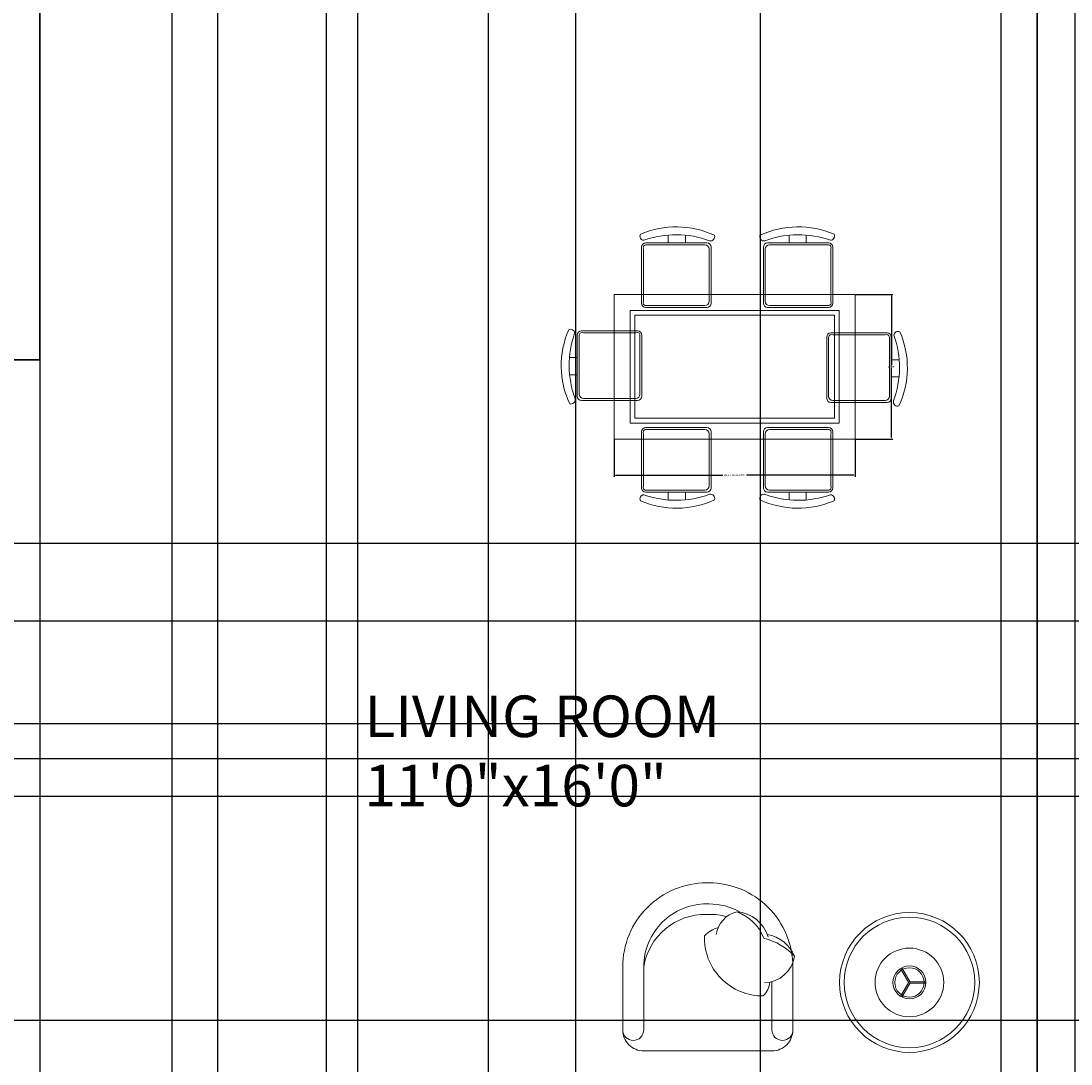
# Model space of a CAD drawing. Units: inches. Extents: x 1861 to 2564, y 1482 to 2317.
# Tile 6 of 11: x 2090 to 2217, y 2018 to 2143. Entities that reach past the tile are written whole.
import ezdxf

# ---------------------------------------------------------------- set-up
doc = ezdxf.new("R2010")
doc.units = ezdxf.units.IN
for name, color, linetype, lineweight in [('A-ANNO-DIMS', 2, 'Continuous', 18), ('A-AREA-IDEN', 7, 'Continuous', 18), ('A-FURN', 8, 'Continuous', 13), ('A-WALL', 7, 'Continuous', 35)]:
    doc.layers.add(name, color=color, linetype=linetype, lineweight=lineweight)
doc.styles.get("Standard").update_dxf_attribs({"font": 'arial.ttf'})
doc.dimstyles.get("Standard").update_dxf_attribs({"dimtxt": 0.18, "dimasz": 0.18, "dimexe": 0.18, "dimexo": 0.0625, "dimgap": 0.09, "dimtad": 0, "dimtih": 1, "dimtoh": 1, "dimdec": 4, "dimzin": 0, "dimdsep": 46, "dimtxsty": 'Standard', "dimcen": 0.09, "dimadec": 0, "dimazin": 0, "dimtfac": 1, "dimtdec": 4, "dimtofl": 0, "dimtmove": 0, "dimatfit": 3, "dimfxl": 1, "dimtolj": 1, "dimtzin": 0, "dimarcsym": 0})

# ---------------------------------------------------------------- blocks, each defined once
blk = doc.blocks.new('TABLE-SIDE-ROUND')
at = {"ltscale": 0.03}
for p, q in [((8.34, 8.45), (9.33, 10.16)), ((8.49, 8.36), (9.48, 10.08)), ((8.41, 8.5), (6.44, 8.5)), ((8.41, 8.32), (6.44, 8.32)), ((8.34, 8.36), (9.33, 6.65)), ((8.49, 8.45), (9.48, 6.74))]:
    blk.add_line(p, q, dxfattribs=at)
for radius in [8.41, 4.13, 1.98, 1.77]:
    blk.add_circle((8.41, 8.41), radius, dxfattribs=at)
blk.add_circle((8.41, 8.41), 7.85)
blk = doc.blocks.new('CHAIR-LOUNGE')
at = {"ltscale": 0.03}
blk.add_lwpolyline([(10.44, 0), (18.15, 0, 0.414214), (20.68, 2.53), (20.68, 10.11, 0.414214), (10.57, 20.22), (10.44, 20.22), (10.32, 20.22, 0.414214), (0.21, 10.11), (0.21, 2.53, 0.414214), (2.73, 0), (10.44, 0)], format="xyb", dxfattribs=at)
for points in [[(6.55, 16.69, -0.130591), (10.32, 17.69), (10.44, 17.69)], [(18.15, 10.11, 0.414214), (10.57, 17.69), (10.44, 17.69)], [(0, 11.38, -0.14773), (3.69, 13.56, -0.213343), (6.95, 16.74, -0.178662)], [(3.18, 13.73, -0.306663), (6.95, 16.74, -0.30633), (9.42, 13.99, 0.872847)], [(8.16, 16.16, -0.072384), (10.32, 16.43), (10.44, 16.43)], [(18.15, 10.11, 0.372719), (10.57, 16.43), (10.44, 16.43)], [(3.62, 8.2, -0.356772), (0, 11.38, -0.249542), (3.28, 14.01, 9.61688)], [(2.98, 8.28, 0.165541), (3.77, 6.61, 0.425989), (10.86, 13.85, 0.121523), (9.18, 14.84, -7.115464)], [(18.15, 10.11), (18.15, 2.53, 0.414214), (19.42, 1.26), (19.42, 1.26, 0.414214), (20.68, 2.53)], [(2.73, 8.34), (2.73, 2.53, -0.414214), (1.47, 1.26), (1.47, 1.26, -0.414214), (0.21, 2.53)]]:
    blk.add_lwpolyline(points, format="xyb")
blk = doc.blocks.new('TABLE-DINING-RECT')
for points in [[(0, 17.4), (29.01, 17.4), (29.01, 0), (0, 0)], [(0, 17.4), (29.01, 17.4), (29.01, 0), (0, 0)], [(1.93, 15.47), (27.08, 15.47), (27.08, 1.93), (1.93, 1.93)], [(1.93, 15.47), (27.08, 15.47), (27.08, 1.93), (1.93, 1.93)], [(2.51, 14.89), (26.5, 14.89), (26.5, 2.51), (2.51, 2.51)], [(2.51, 14.89), (26.5, 14.89), (26.5, 2.51), (2.51, 2.51)]]:
    blk.add_lwpolyline(points, close=True)
blk = doc.blocks.new('*D32')
at = {"layer": 'A-ANNO-DIMS', "color": 0, "lineweight": -2, "transparency": 16777216}
for p, q in [((2161.83, 2092.8), (2161.83, 2088.34)), ((2190.84, 2092.8), (2190.84, 2088.34)), ((2162.01, 2088.52), (2174.9, 2088.52)), ((2190.66, 2088.52), (2177.77, 2088.52))]:
    blk.add_line(p, q, dxfattribs=at)
at = {"layer": 'A-ANNO-DIMS', "color": 0, "transparency": 16777216}
for points in [[(2162.01, 2088.55), (2162.01, 2088.49), (2161.83, 2088.52)], [(2190.66, 2088.55), (2190.66, 2088.49), (2190.84, 2088.52)]]:
    blk.add_solid(points, dxfattribs=at)
at = {"layer": 'Defpoints', "color": 0, "transparency": 16777216}
for p in [(2161.83, 2092.87), (2190.84, 2092.87), (2190.84, 2088.52)]:
    blk.add_point(p, dxfattribs=at)
at = {"layer": 'A-ANNO-DIMS', "color": 0, "transparency": 16777216, "insert": (2176.33, 2088.52), "char_height": 0.18, "attachment_point": 5}
blk.add_mtext('\\A1;DINING TABLE 29 TYP.', dxfattribs=at)
blk = doc.blocks.new('*D33')
at = {"layer": 'A-ANNO-DIMS', "color": 0, "lineweight": -2, "transparency": 16777216}
for p, q in [((2190.9, 2110.27), (2195.37, 2110.27)), ((2195.19, 2110.09), (2195.19, 2101.75)), ((2195.19, 2093.05), (2195.19, 2101.39)), ((2190.9, 2092.87), (2195.37, 2092.87))]:
    blk.add_line(p, q, dxfattribs=at)
at = {"layer": 'A-ANNO-DIMS', "color": 0, "transparency": 16777216}
for points in [[(2195.16, 2110.09), (2195.22, 2110.09), (2195.19, 2110.27)], [(2195.16, 2093.05), (2195.22, 2093.05), (2195.19, 2092.87)]]:
    blk.add_solid(points, dxfattribs=at)
at = {"layer": 'Defpoints', "color": 0, "transparency": 16777216}
for p in [(2190.84, 2110.27), (2195.19, 2110.27), (2190.84, 2092.87)]:
    blk.add_point(p, dxfattribs=at)
at = {"layer": 'A-ANNO-DIMS', "color": 0, "transparency": 16777216, "insert": (2195.19, 2101.57), "char_height": 0.18, "attachment_point": 5}
blk.add_mtext('\\A1;17 TYP.', dxfattribs=at)
blk = doc.blocks.new('*D36')
at = {"layer": 'A-ANNO-DIMS', "color": 0, "lineweight": -2, "transparency": 16777216}
for p, q in [((2092.74, 2250.82), (2092.74, 1545.6)), ((2127.18, 2250.82), (2127.18, 1545.6)), ((2092.92, 1545.78), (2109.5, 1545.78)), ((2127, 1545.78), (2110.43, 1545.78))]:
    blk.add_line(p, q, dxfattribs=at)
at = {"layer": 'A-ANNO-DIMS', "color": 0, "transparency": 16777216}
for points in [[(2092.92, 1545.81), (2092.92, 1545.75), (2092.74, 1545.78)], [(2127, 1545.81), (2127, 1545.75), (2127.18, 1545.78)]]:
    blk.add_solid(points, dxfattribs=at)
at = {"layer": 'Defpoints', "color": 0, "transparency": 16777216}
for p in [(2092.74, 2250.89), (2127.18, 2250.89), (2127.18, 1545.78)]:
    blk.add_point(p, dxfattribs=at)
at = {"layer": 'A-ANNO-DIMS', "color": 0, "transparency": 16777216, "insert": (2109.96, 1545.78), "char_height": 0.18, "attachment_point": 5}
blk.add_mtext('\\A1;34.445', dxfattribs=at)
blk = doc.blocks.new('*D52')
at = {"layer": 'A-ANNO-DIMS', "color": 0, "lineweight": -2, "transparency": 16777216}
for p, q in [((2179.39, 2154.82), (2179.39, 1545.6)), ((2208.37, 2154.82), (2208.37, 1545.6)), ((2179.57, 1545.78), (2193.49, 1545.78)), ((2208.19, 1545.78), (2194.28, 1545.78))]:
    blk.add_line(p, q, dxfattribs=at)
at = {"layer": 'A-ANNO-DIMS', "color": 0, "transparency": 16777216}
for points in [[(2179.57, 1545.81), (2179.57, 1545.75), (2179.39, 1545.78)], [(2208.19, 1545.81), (2208.19, 1545.75), (2208.37, 1545.78)]]:
    blk.add_solid(points, dxfattribs=at)
at = {"layer": 'Defpoints', "color": 0, "transparency": 16777216}
for p in [(2179.39, 2154.89), (2208.37, 2154.89), (2208.37, 1545.78)]:
    blk.add_point(p, dxfattribs=at)
at = {"layer": 'A-ANNO-DIMS', "color": 0, "transparency": 16777216, "insert": (2193.88, 1545.78), "char_height": 0.18, "attachment_point": 5}
blk.add_mtext('\\A1;28.98', dxfattribs=at)
blk = doc.blocks.new('*D55')
at = {"layer": 'A-ANNO-DIMS', "color": 0, "lineweight": -2, "transparency": 16777216}
for p, q in [((2114.18, 1853.45), (2114.18, 2290.37)), ((2114.36, 2290.19), (2130, 2290.19)), ((2146.56, 2290.19), (2130.92, 2290.19)), ((2146.74, 1853.45), (2146.74, 2290.37))]:
    blk.add_line(p, q, dxfattribs=at)
at = {"layer": 'A-ANNO-DIMS', "color": 0, "transparency": 16777216}
for points in [[(2114.36, 2290.22), (2114.36, 2290.16), (2114.18, 2290.19)], [(2146.56, 2290.22), (2146.56, 2290.16), (2146.74, 2290.19)]]:
    blk.add_solid(points, dxfattribs=at)
at = {"layer": 'Defpoints', "color": 0, "transparency": 16777216}
for p in [(2146.74, 2290.19), (2114.18, 1853.39), (2146.74, 1853.39)]:
    blk.add_point(p, dxfattribs=at)
at = {"layer": 'A-ANNO-DIMS', "color": 0, "transparency": 16777216, "insert": (2130.46, 2290.19), "char_height": 0.18, "attachment_point": 5}
blk.add_mtext('\\A1;32.564', dxfattribs=at)
blk = doc.blocks.new('*D61')
at = {"layer": 'A-ANNO-DIMS', "color": 0, "lineweight": -2, "transparency": 16777216}
for p, q in [((2008.8, 2080.33), (2537.22, 2080.33)), ((2537.04, 2080.15), (2537.04, 2069.66)), ((2537.04, 2058.82), (2537.04, 2069.3)), ((2008.8, 2058.64), (2537.22, 2058.64))]:
    blk.add_line(p, q, dxfattribs=at)
at = {"layer": 'A-ANNO-DIMS', "color": 0, "transparency": 16777216}
for points in [[(2537.01, 2080.15), (2537.07, 2080.15), (2537.04, 2080.33)], [(2537.01, 2058.82), (2537.07, 2058.82), (2537.04, 2058.64)]]:
    blk.add_solid(points, dxfattribs=at)
at = {"layer": 'Defpoints', "color": 0, "transparency": 16777216}
for p in [(2008.74, 2080.33), (2537.04, 2080.33), (2008.74, 2058.64)]:
    blk.add_point(p, dxfattribs=at)
at = {"layer": 'A-ANNO-DIMS', "color": 0, "transparency": 16777216, "insert": (2537.04, 2069.48), "char_height": 0.18, "attachment_point": 5}
blk.add_mtext('\\A1;21.693', dxfattribs=at)
blk = doc.blocks.new('*D62')
at = {"layer": 'A-ANNO-DIMS', "color": 0, "lineweight": -2, "transparency": 16777216}
for p, q in [((2108.68, 1781.45), (2108.68, 2290.37)), ((2108.86, 2290.19), (2119.46, 2290.19)), ((2130.84, 2290.19), (2120.25, 2290.19)), ((2131.02, 1781.45), (2131.02, 2290.37))]:
    blk.add_line(p, q, dxfattribs=at)
at = {"layer": 'A-ANNO-DIMS', "color": 0, "transparency": 16777216}
for points in [[(2108.86, 2290.22), (2108.86, 2290.16), (2108.68, 2290.19)], [(2130.84, 2290.22), (2130.84, 2290.16), (2131.02, 2290.19)]]:
    blk.add_solid(points, dxfattribs=at)
at = {"layer": 'Defpoints', "color": 0, "transparency": 16777216}
for p in [(2131.02, 2290.19), (2108.68, 1781.39), (2131.02, 1781.39)]:
    blk.add_point(p, dxfattribs=at)
at = {"layer": 'A-ANNO-DIMS', "color": 0, "transparency": 16777216, "insert": (2119.85, 2290.19), "char_height": 0.18, "attachment_point": 5}
blk.add_mtext('\\A1;22.34', dxfattribs=at)
blk = doc.blocks.new('*D64')
at = {"layer": 'A-ANNO-DIMS', "color": 0, "lineweight": -2, "transparency": 16777216}
for p, q in [((2497.68, 2070.96), (1892.76, 2070.96)), ((1892.94, 2070.78), (1892.94, 2062.85)), ((1892.94, 2054.57), (1892.94, 2062.49)), ((2497.68, 2054.39), (1892.76, 2054.39))]:
    blk.add_line(p, q, dxfattribs=at)
at = {"layer": 'A-ANNO-DIMS', "color": 0, "transparency": 16777216}
for points in [[(1892.91, 2070.78), (1892.97, 2070.78), (1892.94, 2070.96)], [(1892.91, 2054.57), (1892.97, 2054.57), (1892.94, 2054.39)]]:
    blk.add_solid(points, dxfattribs=at)
at = {"layer": 'Defpoints', "color": 0, "transparency": 16777216}
for p in [(2497.74, 2070.96), (1892.94, 2054.39), (2497.74, 2054.39)]:
    blk.add_point(p, dxfattribs=at)
at = {"layer": 'A-ANNO-DIMS', "color": 0, "transparency": 16777216, "insert": (1892.94, 2062.67), "char_height": 0.18, "attachment_point": 5}
blk.add_mtext('\\A1;16.57', dxfattribs=at)
blk = doc.blocks.new('*D65')
at = {"layer": 'A-ANNO-DIMS', "color": 0, "lineweight": -2, "transparency": 16777216}
for p, q in [((2497.68, 2049.89), (1892.76, 2049.89)), ((1892.94, 2049.71), (1892.94, 2036.58)), ((1892.94, 2023.09), (1892.94, 2036.22)), ((2497.68, 2022.91), (1892.76, 2022.91))]:
    blk.add_line(p, q, dxfattribs=at)
at = {"layer": 'A-ANNO-DIMS', "color": 0, "transparency": 16777216}
for points in [[(1892.91, 2049.71), (1892.97, 2049.71), (1892.94, 2049.89)], [(1892.91, 2023.09), (1892.97, 2023.09), (1892.94, 2022.91)]]:
    blk.add_solid(points, dxfattribs=at)
at = {"layer": 'Defpoints', "color": 0, "transparency": 16777216}
for p in [(2497.74, 2049.89), (1892.94, 2022.91), (2497.74, 2022.91)]:
    blk.add_point(p, dxfattribs=at)
at = {"layer": 'A-ANNO-DIMS', "color": 0, "transparency": 16777216, "insert": (1892.94, 2036.4), "char_height": 0.18, "attachment_point": 5}
blk.add_mtext('\\A1;26.973', dxfattribs=at)
blk = doc.blocks.new('*D68')
at = {"layer": 'A-ANNO-DIMS', "color": 0, "lineweight": -2, "transparency": 16777216}
for p, q in [((2157.24, 1794.95), (2157.24, 2290.37)), ((2157.42, 2290.19), (2184.66, 2290.19)), ((2212.56, 2290.19), (2185.31, 2290.19)), ((2212.74, 1794.95), (2212.74, 2290.37))]:
    blk.add_line(p, q, dxfattribs=at)
at = {"layer": 'A-ANNO-DIMS', "color": 0, "transparency": 16777216}
for points in [[(2157.42, 2290.22), (2157.42, 2290.16), (2157.24, 2290.19)], [(2212.56, 2290.22), (2212.56, 2290.16), (2212.74, 2290.19)]]:
    blk.add_solid(points, dxfattribs=at)
at = {"layer": 'Defpoints', "color": 0, "transparency": 16777216}
for p in [(2212.74, 2290.19), (2157.24, 1794.89), (2212.74, 1794.89)]:
    blk.add_point(p, dxfattribs=at)
at = {"layer": 'A-ANNO-DIMS', "color": 0, "transparency": 16777216, "insert": (2184.99, 2290.19), "char_height": 0.18, "attachment_point": 5}
blk.add_mtext('\\A1;55.5', dxfattribs=at)
blk = doc.blocks.new('*D71')
at = {"layer": 'A-ANNO-DIMS', "color": 0, "lineweight": -2, "transparency": 16777216}
for p, q in [((2212.74, 2250.82), (2212.74, 1545.6)), ((2217.24, 2250.82), (2217.24, 1545.6)), ((2212.92, 1545.78), (2214.73, 1545.78)), ((2217.06, 1545.78), (2215.25, 1545.78))]:
    blk.add_line(p, q, dxfattribs=at)
at = {"layer": 'A-ANNO-DIMS', "color": 0, "transparency": 16777216}
for points in [[(2212.92, 1545.81), (2212.92, 1545.75), (2212.74, 1545.78)], [(2217.06, 1545.81), (2217.06, 1545.75), (2217.24, 1545.78)]]:
    blk.add_solid(points, dxfattribs=at)
at = {"layer": 'Defpoints', "color": 0, "transparency": 16777216}
for p in [(2212.74, 2250.89), (2217.24, 2250.89), (2217.24, 1545.78)]:
    blk.add_point(p, dxfattribs=at)
at = {"layer": 'A-ANNO-DIMS', "color": 0, "transparency": 16777216, "insert": (2214.99, 1545.78), "char_height": 0.18, "attachment_point": 5}
blk.add_mtext('\\A1;4.5', dxfattribs=at)

msp = doc.modelspace()

# ---------------------------------------------------------------- linework, layer by layer
at = {"layer": 'A-FURN'}
for points in [[(2165.4177, 2116.7864, -0.17580919), (2173.3194, 2116.7265, 0.57839206), (2173.918, 2117.3847, 0.21452438), (2164.9987, 2117.5044, 0.55201397), (2165.4177, 2116.7864, -0.06507904)], [(2165.4177, 2116.7861, -0.17580919), (2173.3194, 2116.7262, 0.57839206), (2173.9181, 2117.3844, 0.21452438), (2164.9987, 2117.5041, 0.55201397), (2165.4177, 2116.7861, -0.06507904)], [(2179.9716, 2116.7265, -0.57839206), (2179.373, 2117.3847, -0.21452438), (2188.2924, 2117.5044, -0.55201397), (2187.8733, 2116.7864, 0.1758092), (2179.9716, 2116.7265)], [(2179.9717, 2116.7262, -0.57839206), (2179.373, 2117.3844, -0.21452438), (2188.2924, 2117.5041, -0.55201397), (2187.8734, 2116.7861, 0.1758092), (2179.9717, 2116.7262)], [(2170.4075, 2116.4692), (2170.4075, 2117.397, -0.06475861)], [(2170.4076, 2116.4689), (2170.4076, 2117.3967, -0.06475861)], [(2182.8835, 2116.4692), (2182.8835, 2117.397, 0.06475861)], [(2182.8835, 2116.4689), (2182.8835, 2117.3967, 0.06475861)], [(2172.9842, 2116.4692), (2165.6485, 2116.4692, 0.41421356), (2165.1353, 2115.956), (2165.1353, 2109.211, 0.41421356), (2165.6485, 2108.6978), (2172.9842, 2108.6978, 0.41421356), (2173.4974, 2109.211), (2173.4974, 2115.956, 0.41421356), (2172.9842, 2116.4692)], [(2172.9842, 2116.4689), (2165.6485, 2116.4689, 0.41421356), (2165.1353, 2115.9557), (2165.1353, 2109.2107, 0.41421356), (2165.6485, 2108.6975), (2172.9842, 2108.6975, 0.41421356), (2173.4974, 2109.2107), (2173.4974, 2115.9557, 0.41421356), (2172.9842, 2116.4689)], [(2187.6425, 2116.4692, -0.41421356), (2188.1558, 2115.956), (2188.1558, 2109.211, -0.41421356), (2187.6425, 2108.6978), (2180.3069, 2108.6978, -0.41421356), (2179.7937, 2109.211), (2179.7937, 2115.956, -0.41421356), (2180.3069, 2116.4692), (2187.6425, 2116.4692)], [(2187.6426, 2116.4689, -0.41421356), (2188.1558, 2115.9557), (2188.1558, 2109.2107, -0.41421356), (2187.6426, 2108.6975), (2180.3069, 2108.6975, -0.41421356), (2179.7937, 2109.2107), (2179.7937, 2115.9557, -0.41421356), (2180.3069, 2116.4689), (2187.6426, 2116.4689)], [(2157.151, 2097.7049, -0.57839206), (2156.4928, 2097.1063, -0.21452438), (2156.3731, 2106.0257, -0.55201397), (2157.0912, 2105.6066, 0.17580937), (2157.151, 2097.7049)], [(2157.151, 2097.7046, -0.57839206), (2156.4928, 2097.106, -0.21452438), (2156.3731, 2106.0254, -0.55201397), (2157.0912, 2105.6063, 0.17580937), (2157.151, 2097.7046)], [(2157.4083, 2105.3759, -0.41421356), (2157.9215, 2105.8891), (2164.6665, 2105.8891, -0.41421356), (2165.1798, 2105.3759), (2165.1798, 2098.0402, -0.41421356), (2164.6665, 2097.527), (2157.9215, 2097.527, -0.41421356), (2157.4083, 2098.0402), (2157.4083, 2105.3759)], [(2157.4083, 2105.3755, -0.41421356), (2157.9216, 2105.8888), (2164.6666, 2105.8888, -0.41421356), (2165.1798, 2105.3755), (2165.1798, 2098.0399, -0.41421356), (2164.6666, 2097.5267), (2157.9216, 2097.5267, -0.41421356), (2157.4083, 2098.0399), (2157.4083, 2105.3755)], [(2195.1836, 2105.1246, 0.41421356), (2194.6704, 2105.6378), (2187.9254, 2105.6378, 0.41421356), (2187.4122, 2105.1246), (2187.4122, 2097.7889, 0.41421356), (2187.9254, 2097.2757), (2194.6704, 2097.2757, 0.41421356), (2195.1836, 2097.7889), (2195.1836, 2105.1246)], [(2195.1836, 2105.1243, 0.41421356), (2194.6704, 2105.6375), (2187.9254, 2105.6375, 0.41421356), (2187.4122, 2105.1243), (2187.4122, 2097.7886, 0.41421356), (2187.9254, 2097.2754), (2194.6704, 2097.2754, 0.41421356), (2195.1836, 2097.7886), (2195.1836, 2105.1243)], [(2195.5007, 2105.3554, -0.17580919), (2195.4409, 2097.4537, 0.57839206), (2196.0991, 2096.8551, 0.21452438), (2196.2188, 2105.7744, 0.55201397), (2195.5007, 2105.3554, -0.06507904)], [(2195.5008, 2105.3551, -0.17580919), (2195.4409, 2097.4534, 0.57839206), (2196.0991, 2096.8548, 0.21452438), (2196.2188, 2105.7741, 0.55201397), (2195.5008, 2105.3551, -0.06507904)], [(2157.4083, 2100.6168), (2156.4806, 2100.6168, 0.06475861)], [(2157.4083, 2100.6165), (2156.4806, 2100.6165, 0.06475861)], [(2195.1836, 2100.3656), (2196.1113, 2100.3656, -0.06475861)], [(2195.1836, 2100.3653), (2196.1114, 2100.3653, -0.06475861)], [(2172.9842, 2086.486), (2165.6485, 2086.486, -0.41421356), (2165.1353, 2086.9992), (2165.1353, 2093.7442, -0.41421356), (2165.6485, 2094.2574), (2172.9842, 2094.2574, -0.41421356), (2173.4974, 2093.7442), (2173.4974, 2086.9992, -0.41421356), (2172.9842, 2086.486)], [(2172.9842, 2086.4857), (2165.6485, 2086.4857, -0.41421356), (2165.1353, 2086.9989), (2165.1353, 2093.7439, -0.41421356), (2165.6485, 2094.2571), (2172.9842, 2094.2571, -0.41421356), (2173.4974, 2093.7439), (2173.4974, 2086.9989, -0.41421356), (2172.9842, 2086.4857)], [(2187.6425, 2086.486, 0.41421356), (2188.1558, 2086.9992), (2188.1558, 2093.7442, 0.41421356), (2187.6425, 2094.2574), (2180.3069, 2094.2574, 0.41421356), (2179.7937, 2093.7442), (2179.7937, 2086.9992, 0.41421356), (2180.3069, 2086.486), (2187.6425, 2086.486)], [(2187.6426, 2086.4857, 0.41421356), (2188.1558, 2086.9989), (2188.1558, 2093.7439, 0.41421356), (2187.6426, 2094.2571), (2180.3069, 2094.2571, 0.41421356), (2179.7937, 2093.7439), (2179.7937, 2086.9989, 0.41421356), (2180.3069, 2086.4857), (2187.6426, 2086.4857)], [(2173.3194, 2086.2287, -0.57839206), (2173.918, 2085.5705, -0.21452438), (2164.9987, 2085.4508, -0.55201397), (2165.4177, 2086.1689, 0.17580929), (2173.3194, 2086.2287)], [(2173.3194, 2086.2284, -0.57839206), (2173.9181, 2085.5702, -0.21452438), (2164.9987, 2085.4505, -0.55201397), (2165.4177, 2086.1686, 0.17580929), (2173.3194, 2086.2284)], [(2170.4075, 2086.486), (2170.4075, 2085.5583, 0.06475861)], [(2170.4076, 2086.4857), (2170.4076, 2085.558, 0.06475861)], [(2187.8733, 2086.1689, -0.17580928), (2179.9716, 2086.2287, 0.57839206), (2179.373, 2085.5705, 0.21452438), (2188.2924, 2085.4508, 0.55201397), (2187.8733, 2086.1689, -0.06507904)], [(2187.8734, 2086.1686, -0.17580928), (2179.9717, 2086.2284, 0.57839206), (2179.373, 2085.5702, 0.21452438), (2188.2924, 2085.4505, 0.55201397), (2187.8734, 2086.1686, -0.06507904)], [(2182.8835, 2086.486), (2182.8835, 2085.5583, -0.06475861)], [(2182.8835, 2086.4857), (2182.8835, 2085.558, -0.06475861)]]:
    msp.add_lwpolyline(points, format="xyb", dxfattribs=at)
for points in [[(2168.3542, 2117.4138), (2168.3542, 2116.4692)], [(2168.3542, 2117.4135), (2168.3542, 2116.4689)], [(2184.9369, 2117.4138), (2184.9369, 2116.4692)], [(2184.9369, 2117.4135), (2184.9369, 2116.4689)], [(2156.4637, 2102.6702), (2157.4083, 2102.6702)], [(2156.4637, 2102.6699), (2157.4083, 2102.6699)], [(2196.1282, 2102.419), (2195.1836, 2102.419)], [(2196.1282, 2102.4187), (2195.1836, 2102.4187)], [(2168.3542, 2085.5414), (2168.3542, 2086.486)], [(2168.3542, 2085.5411), (2168.3542, 2086.4857)], [(2184.9369, 2085.5414), (2184.9369, 2086.486)], [(2184.9369, 2085.5411), (2184.9369, 2086.4857)]]:
    msp.add_lwpolyline(points, dxfattribs=at)
for points in [[(2165.6516, 2116.238), (2172.753, 2116.238, -0.41421356), (2173.2662, 2115.7248), (2173.2662, 2109.4422, -0.41421356), (2172.753, 2108.929), (2165.6516, 2108.929, -0.51206948), (2165.3665, 2109.4422), (2165.3665, 2115.7248, -0.51206948)], [(2165.6516, 2116.2377), (2172.753, 2116.2377, -0.41421356), (2173.2662, 2115.7245), (2173.2662, 2109.4419, -0.41421356), (2172.753, 2108.9287), (2165.6516, 2108.9287, -0.51206948), (2165.3665, 2109.4419), (2165.3665, 2115.7245, -0.51206948)], [(2187.6394, 2116.238), (2180.5381, 2116.238, 0.41421356), (2180.0249, 2115.7248), (2180.0249, 2109.4422, 0.41421356), (2180.5381, 2108.929), (2187.6394, 2108.929, 0.51206948), (2187.9246, 2109.4422), (2187.9246, 2115.7248, 0.51206948)], [(2187.6395, 2116.2377), (2180.5381, 2116.2377, 0.41421356), (2180.0249, 2115.7245), (2180.0249, 2109.4419, 0.41421356), (2180.5381, 2108.9287), (2187.6395, 2108.9287, 0.51206948), (2187.9246, 2109.4419), (2187.9246, 2115.7245, 0.51206948)], [(2157.6395, 2105.3727), (2157.6395, 2098.2714, 0.41421356), (2158.1527, 2097.7582), (2164.4353, 2097.7582, 0.41421356), (2164.9486, 2098.2714), (2164.9486, 2105.3727, 0.51206948), (2164.4353, 2105.6579), (2158.1527, 2105.6579, 0.51206948)], [(2157.6395, 2105.3724), (2157.6395, 2098.2711, 0.41421356), (2158.1528, 2097.7579), (2164.4354, 2097.7579, 0.41421356), (2164.9486, 2098.2711), (2164.9486, 2105.3724, 0.51206948), (2164.4354, 2105.6576), (2158.1528, 2105.6576, 0.51206948)], [(2194.9524, 2105.1215), (2194.9524, 2098.0202, -0.41421356), (2194.4392, 2097.5069), (2188.1566, 2097.5069, -0.41421356), (2187.6434, 2098.0202), (2187.6434, 2105.1215, -0.51206948), (2188.1566, 2105.4066), (2194.4392, 2105.4066, -0.51206948)], [(2194.9524, 2105.1212), (2194.9524, 2098.0198, -0.41421356), (2194.4392, 2097.5066), (2188.1566, 2097.5066, -0.41421356), (2187.6434, 2098.0198), (2187.6434, 2105.1212, -0.51206948), (2188.1566, 2105.4063), (2194.4392, 2105.4063, -0.51206948)], [(2165.6516, 2086.7172), (2172.753, 2086.7172, 0.41421356), (2173.2662, 2087.2304), (2173.2662, 2093.513, 0.41421356), (2172.753, 2094.0262), (2165.6516, 2094.0262, 0.51206948), (2165.3665, 2093.513), (2165.3665, 2087.2304, 0.51206948)], [(2165.6516, 2086.7169), (2172.753, 2086.7169, 0.41421356), (2173.2662, 2087.2301), (2173.2662, 2093.5127, 0.41421356), (2172.753, 2094.0259), (2165.6516, 2094.0259, 0.51206948), (2165.3665, 2093.5127), (2165.3665, 2087.2301, 0.51206948)], [(2187.6394, 2086.7172), (2180.5381, 2086.7172, -0.41421356), (2180.0249, 2087.2304), (2180.0249, 2093.513, -0.41421356), (2180.5381, 2094.0262), (2187.6394, 2094.0262, -0.51206948), (2187.9246, 2093.513), (2187.9246, 2087.2304, -0.51206948)], [(2187.6395, 2086.7169), (2180.5381, 2086.7169, -0.41421356), (2180.0249, 2087.2301), (2180.0249, 2093.5127, -0.41421356), (2180.5381, 2094.0259), (2187.6395, 2094.0259, -0.51206948), (2187.9246, 2093.5127), (2187.9246, 2087.2301, -0.51206948)]]:
    msp.add_lwpolyline(points, format="xyb", close=True, dxfattribs=at)
at = {"layer": 'A-WALL'}
for p, q in [((2092.7393, 2250.8854), (2092.7393, 2102.3854)), ((2212.7393, 2150.3854), (2212.7393, 1873.6681)), ((2081.9034, 2102.3854), (2092.7393, 2102.3854))]:
    msp.add_line(p, q, dxfattribs=at)

# ---------------------------------------------------------------- block references
at = {"layer": 'A-FURN'}
msp.add_blockref('TABLE-DINING-RECT', (2161.83, 2092.87), dxfattribs=at)
at = {"layer": 'A-FURN', "extrusion": (0, 0, -1), "zscale": -1}
msp.add_blockref('CHAIR-LOUNGE', (-2183.5533, 2019.2655), dxfattribs=at)
at = {"layer": 'A-FURN', "rotation": 180}
msp.add_blockref('TABLE-SIDE-ROUND', (2205.7733, 2035.9123), dxfattribs=at)

# ---------------------------------------------------------------- texts
at = {"layer": 'A-AREA-IDEN', "insert": (2131.8092, 2062.0191), "char_height": 5, "attachment_point": 1}
msp.add_mtext_dynamic_manual_height_columns('LIVING ROOM\\P11\'0"x16\'0"', width=138.970895, gutter_width=12.5, heights=[0], dxfattribs=at)

# ---------------------------------------------------------------- dimensions: what is measured, and where the dimension line sits
at = {"layer": 'A-ANNO-DIMS'}
for base, p1, p2, override, picture, middle in [((2131.0193, 2290.1854), (2108.6812, 1781.3854), (2131.0193, 1781.3854), {"dimdec": 2, "dimlfac": 1, "dimrnd": 0, "dimzin": 0, "dimdsep": 46, "dimlunit": 2}, '*D62', (2119.8502, 2290.1854)), ((2146.7425, 2290.1854), (2114.1781, 1853.3854), (2146.7425, 1853.3854), {"dimdec": 3, "dimlfac": 1, "dimrnd": 0, "dimzin": 0, "dimdsep": 46, "dimlunit": 2}, '*D55', (2130.4603, 2290.1854)), ((2212.7393, 2290.1854), (2157.2393, 1794.8854), (2212.7393, 1794.8854), {"dimdec": 1, "dimlfac": 1, "dimrnd": 0, "dimzin": 0, "dimdsep": 46, "dimlunit": 2}, '*D68', (2184.9893, 2290.1854)), ((2127.1841, 1545.7777), (2092.7393, 2250.8854), (2127.1841, 2250.8854), {"dimdec": 3, "dimlfac": 1, "dimrnd": 0, "dimzin": 0, "dimdsep": 46, "dimlunit": 2}, '*D36', (2109.9617, 1545.7777)), ((2217.2393, 1545.7777), (2212.7393, 2250.8854), (2217.2393, 2250.8854), {"dimdec": 1, "dimlfac": 1, "dimrnd": 0, "dimzin": 0, "dimdsep": 46, "dimlunit": 2}, '*D71', (2214.9893, 1545.7777)), ((2208.3728, 1545.7777), (2179.3907, 2154.8854), (2208.3728, 2154.8854), {"dimdec": 2, "dimlfac": 1, "dimrnd": 0, "dimzin": 0, "dimdsep": 46, "dimlunit": 2}, '*D52', (2193.8817, 1545.7777))]:
    dim = msp.add_linear_dim(base=base, p1=p1, p2=p2, dimstyle='Standard', override=override, dxfattribs=at)
    dim.commit()
    dim.dimension.update_dxf_attribs({"geometry": picture, "text_midpoint": middle})
dim = msp.add_linear_dim(base=(2195.1918, 2110.2741), p1=(2190.8402, 2092.8673), p2=(2190.8402, 2110.2741), angle=90, text='<> TYP.', dimstyle='Standard', override={"dimdec": 0, "dimlfac": 1, "dimrnd": 0, "dimzin": 0, "dimdsep": 46, "dimlunit": 2}, dxfattribs=at)
dim.commit()
dim.dimension.update_dxf_attribs({"geometry": '*D33', "text_midpoint": (2195.1918, 2101.5707)})
dim = msp.add_linear_dim(base=(2190.8402, 2088.5157), p1=(2161.8294, 2092.8673), p2=(2190.8402, 2092.8673), text='DINING TABLE <> TYP.', dimstyle='Standard', override={"dimdec": 0, "dimlfac": 1, "dimrnd": 0, "dimzin": 0, "dimdsep": 46, "dimlunit": 2}, dxfattribs=at)
dim.commit()
dim.dimension.update_dxf_attribs({"geometry": '*D32', "text_midpoint": (2176.3348, 2088.5157)})
for base, p1, p2, override, picture, middle in [((2537.0393, 2080.3283), (2008.7393, 2058.6356), (2008.7393, 2080.3283), {"dimdec": 3, "dimlfac": 1, "dimrnd": 0, "dimzin": 0, "dimdsep": 46, "dimlunit": 2}, '*D61', (2537.0393, 2069.4819)), ((1892.9393, 2054.3854), (2497.7393, 2070.957), (2497.7393, 2054.3854), {"dimdec": 2, "dimlfac": 1, "dimrnd": 0, "dimzin": 0, "dimdsep": 46, "dimlunit": 2}, '*D64', (1892.9393, 2062.6712)), ((1892.9393, 2022.9123), (2497.7393, 2049.8854), (2497.7393, 2022.9123), {"dimdec": 3, "dimlfac": 1, "dimrnd": 0, "dimzin": 0, "dimdsep": 46, "dimlunit": 2}, '*D65', (1892.9393, 2036.3989))]:
    dim = msp.add_linear_dim(base=base, p1=p1, p2=p2, angle=90, dimstyle='Standard', override=override, dxfattribs=at)
    dim.commit()
    dim.dimension.update_dxf_attribs({"geometry": picture, "text_midpoint": middle})

doc.saveas('drawing.dxf')
